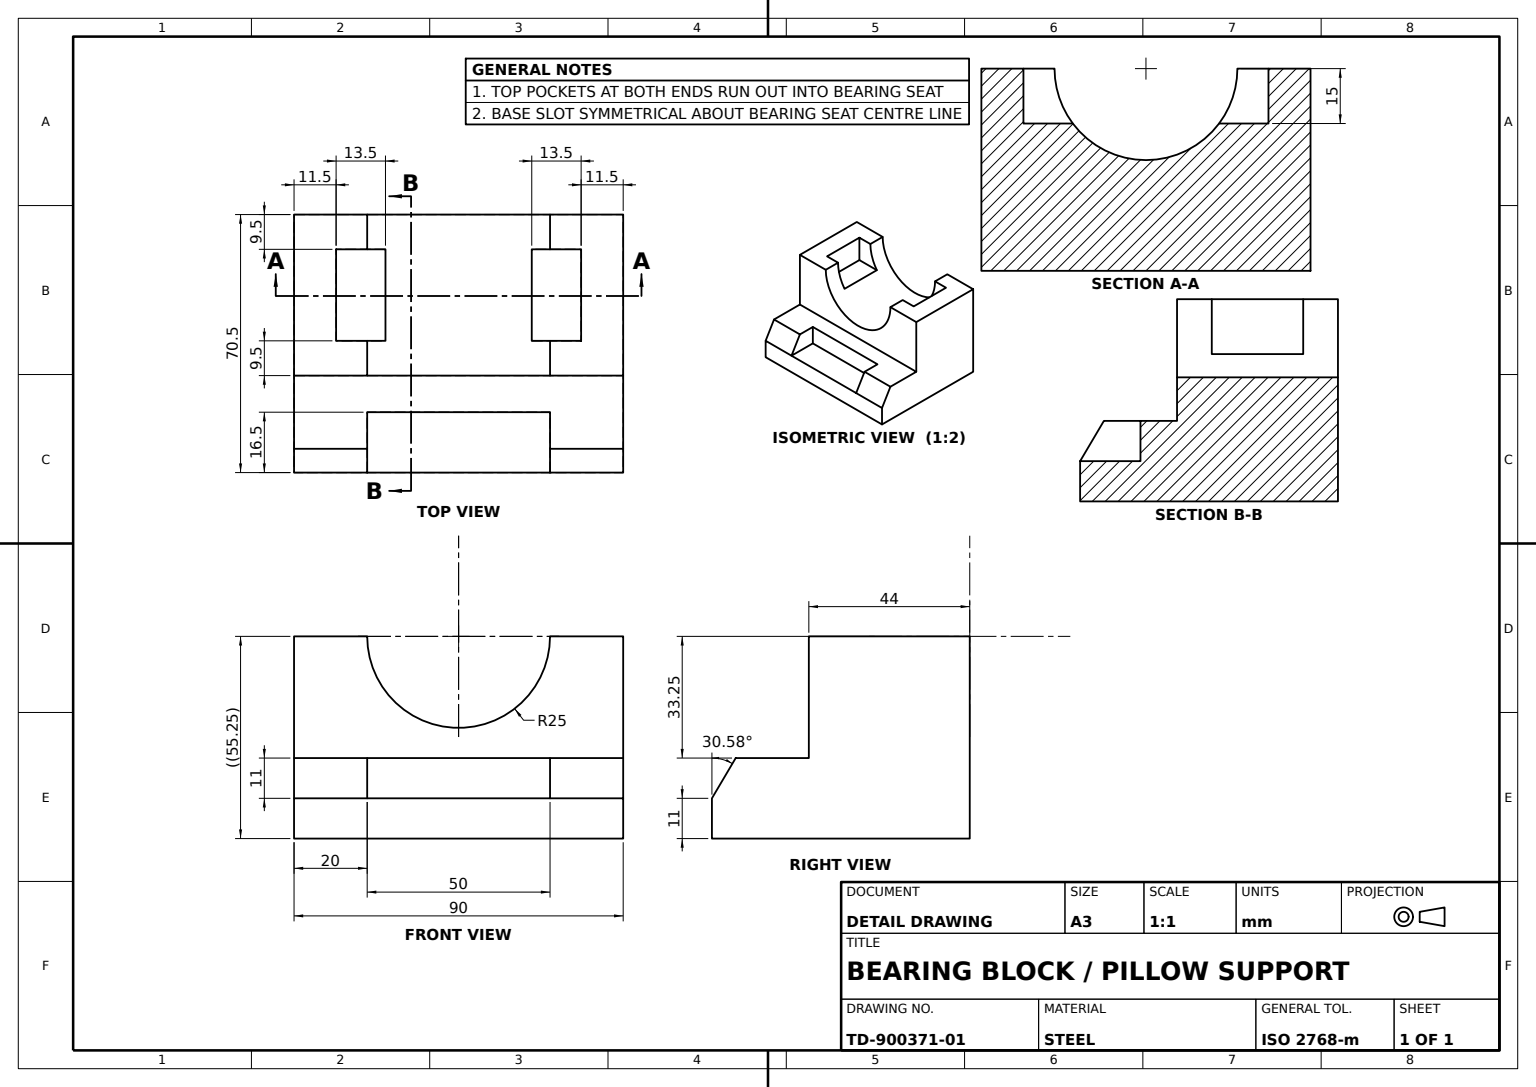
SolidWorks part; units mm, degrees
material "Plain Carbon Steel"
ref_plane "Front Plane" through (0, 0, 0) normal (0, 0, 1) x (1, 0, 0)
ref_plane "Top Plane" through (0, 0, 0) normal (0, 1, 0) x (1, 0, 0)
ref_plane "Right Plane" through (0, 0, 0) normal (1, 0, 0) x (0, 0, -1)
sketch "Bracket Profile Sketch" plane through (0, 0, 0) normal (0, 0, 1) x (1, 0, 0)
  line L0 (0, 0) -> (44, 0)
  line L1 (44, 0) -> (44, 55.25)
  line L2 (44, 55.25) -> (0, 55.25)
  line L3 (0, 55.25) -> (0, 0)
  line L4 (44, 0) -> (70.5, 0)
  line L5 (70.5, 0) -> (70.5, 11)
  line L6 (44, 55.25) -> (44, 22) construction
  line L7 (44, 22) -> (64, 22)
  line L8 (64, 22) -> (70.5, 11)
  dimension "D1" = 70.5
  dimension "D2" = 44
  dimension "D3" = 33.25
  dimension "D4" = 20
  dimension "D5" = 11
  dimension "D6" = 55.25
extrude "Bracket Body" add sketch "Bracket Profile Sketch" along normal mid plane 90 contours L2 L3 L0 L1 | L8 L7 L1 L4 L5
sketch "Bearing Seat Sketch" plane through (44, 0, 0) normal (1, 0, 0) x (0, 0, -1)
  line L0 (-45, 55.25) -> (45, 55.25) construction
  line L1 (-25, 55.25) -> (25, 55.25)
  arc A0 (-25, 55.25) -> (25, 55.25) centre (0, 55.25) ccw
  dimension "D1" = 25
extrude "Bearing Seat R25" cut sketch "Bearing Seat Sketch" against normal blind 45
sketch "Base Slot Sketch" plane through (0, 22, 0) normal (0, 1, 0) x (1, 0, 0)
  line L2 (54, -25) -> (54, 25)
  line L3 (54, 25) -> (70.5, 25)
  line L4 (70.5, -45) -> (70.5, 45) construction
  line L5 (70.5, 25) -> (70.5, -25)
  line L6 (70.5, -25) -> (54, -25)
  dimension "D1" = 16.5
  dimension "D2" = 50
  dimension "D3" = 25
extrude "Base Mounting Slot" cut sketch "Base Slot Sketch" against normal blind 11
sketch "Top Recess Sketch" plane through (0, 55.25, 0) normal (0, 1, 0) x (1, 0, 0)
  line L0 (44, 45) -> (0, 45) construction
  line L3 (0, 25) -> (0, 45) construction
  line L5 (9.5, -33.5) -> (22, -33.5)
  line L7 (22, 33.5) -> (34.5, 33.5)
  line L8 (34.5, 33.5) -> (34.5, 18.5)
  line L9 (34.5, 18.5) -> (9.5, 18.5)
  line L10 (9.5, 18.5) -> (9.5, 33.5)
  line L11 (9.5, 33.5) -> (22, 33.5)
  line L12 (0, 0) -> (44, 0) construction
  line L13 (0, 25) -> (0, -25) construction
  line L14 (44, -45) -> (44, 45) construction
  line L15 (9.5, -18.5) -> (9.5, -33.5)
  line L16 (34.5, -18.5) -> (9.5, -18.5)
  line L17 (34.5, -33.5) -> (34.5, -18.5)
  line L18 (22, -33.5) -> (34.5, -33.5)
  dimension "D1" = 12.5
  dimension "D2" = 25
  dimension "D3" = 15
  dimension "D4" = 11.5
  dimension "D5" = 15
  dimension "D6" = 9.5
extrude "Top Recesses" cut sketch "Top Recess Sketch" against normal blind 15
